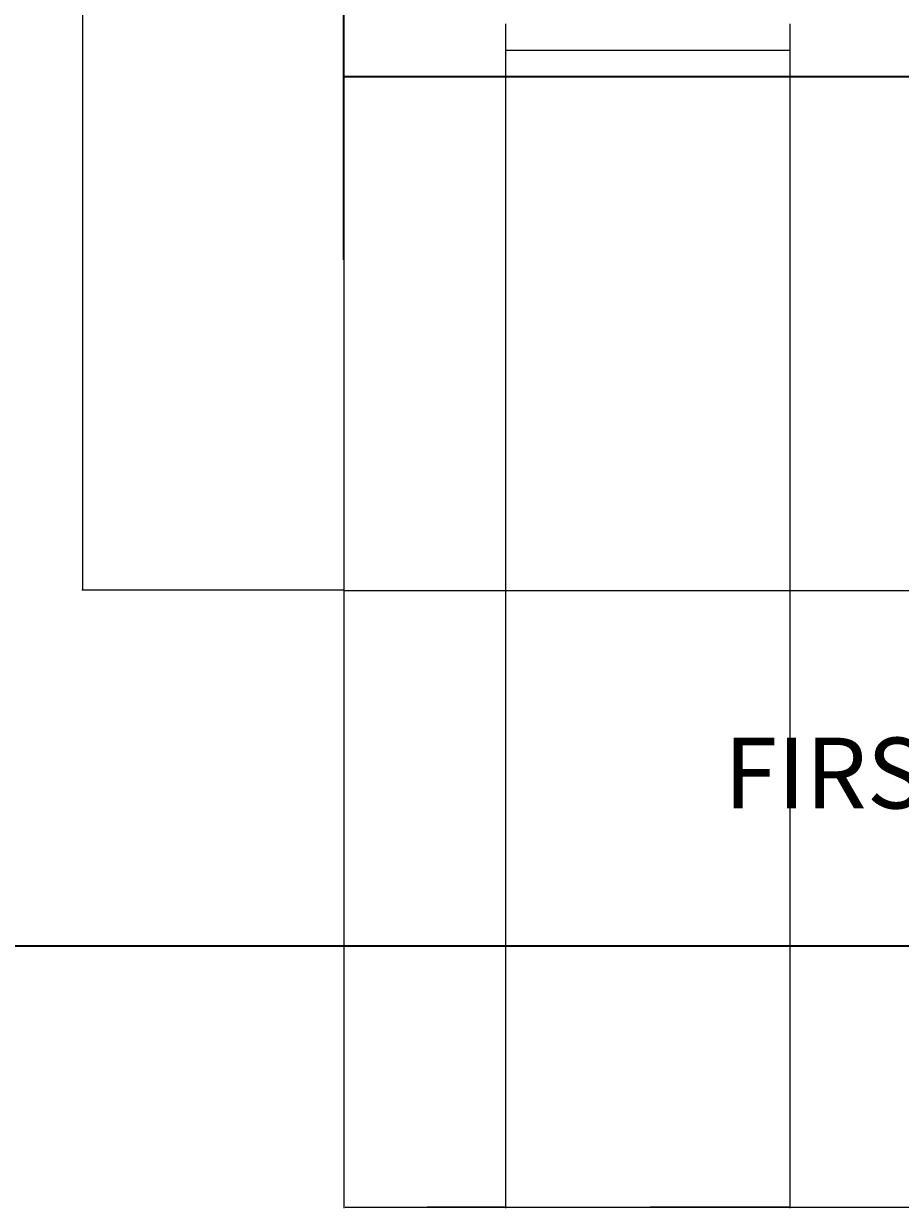
# Model space of a CAD drawing. Units: feet. Extents: x 2100 to 2836, y 2433 to 3396.
# Tile 2 of 12: x 2468 to 2616, y 2433 to 2634. Entities that reach past the tile are written whole.
import ezdxf

# ---------------------------------------------------------------- set-up
doc = ezdxf.new("R2010")
doc.units = ezdxf.units.FT
for name, color, linetype, lineweight in [('A-ANNO-DIMS', 2, 'Continuous', 18), ('A-ANNO-TITL', 7, 'Continuous', 25), ('A-ANNO-TTLB', 7, 'Continuous', 35), ('A-GLAZ', 4, 'Continuous', 18), ('A-WALL', 7, 'Continuous', 35), ('C-PROP', 8, 'Continuous', 18)]:
    doc.layers.add(name, color=color, linetype=linetype, lineweight=lineweight)
doc.styles.get("Standard").update_dxf_attribs({"font": 'arial.ttf'})
doc.dimstyles.get("Standard").update_dxf_attribs({"dimtxt": 0.18, "dimasz": 0.18, "dimexe": 0.18, "dimexo": 0.0625, "dimgap": 0.09, "dimtad": 0, "dimtih": 1, "dimtoh": 1, "dimdec": 4, "dimzin": 0, "dimdsep": 46, "dimtxsty": 'Standard', "dimcen": 0.09, "dimadec": 0, "dimazin": 0, "dimtfac": 1, "dimtdec": 4, "dimtofl": 0, "dimtmove": 0, "dimatfit": 3, "dimfxl": 1, "dimtolj": 1, "dimtzin": 0, "dimarcsym": 0})

# ---------------------------------------------------------------- blocks, each defined once
blk = doc.blocks.new('*D42')
at = {"layer": 'A-ANNO-DIMS', "color": 0, "lineweight": -2, "transparency": 16777216}
for p, q in [((2521.95, 2537.69), (2521.95, 2433.01)), ((2740.95, 2537.69), (2740.95, 2433.01)), ((2522.13, 2433.19), (2631.16, 2433.19)), ((2740.77, 2433.19), (2631.74, 2433.19))]:
    blk.add_line(p, q, dxfattribs=at)
at = {"layer": 'A-ANNO-DIMS', "color": 0, "transparency": 16777216}
for points in [[(2522.13, 2433.22), (2522.13, 2433.16), (2521.95, 2433.19)], [(2740.77, 2433.22), (2740.77, 2433.16), (2740.95, 2433.19)]]:
    blk.add_solid(points, dxfattribs=at)
at = {"layer": 'Defpoints', "color": 0, "transparency": 16777216}
for p in [(2521.95, 2537.76), (2740.95, 2537.76), (2740.95, 2433.19)]:
    blk.add_point(p, dxfattribs=at)
at = {"layer": 'A-ANNO-DIMS', "color": 0, "transparency": 16777216, "insert": (2631.45, 2433.19), "char_height": 0.18, "attachment_point": 5}
blk.add_mtext('\\A1;219', dxfattribs=at)
blk = doc.blocks.new('*D43')
at = {"layer": 'A-ANNO-DIMS', "color": 0, "lineweight": -2, "transparency": 16777216}
for p, q in [((2521.89, 3321.8), (2477.52, 3321.8)), ((2477.7, 3321.62), (2477.7, 2929.96)), ((2477.7, 2537.94), (2477.7, 2929.6)), ((2521.89, 2537.76), (2477.52, 2537.76))]:
    blk.add_line(p, q, dxfattribs=at)
at = {"layer": 'A-ANNO-DIMS', "color": 0, "transparency": 16777216}
for points in [[(2477.67, 3321.62), (2477.73, 3321.62), (2477.7, 3321.8)], [(2477.67, 2537.94), (2477.73, 2537.94), (2477.7, 2537.76)]]:
    blk.add_solid(points, dxfattribs=at)
at = {"layer": 'Defpoints', "color": 0, "transparency": 16777216}
for p in [(2477.7, 3321.8), (2521.95, 3321.8), (2521.95, 2537.76)]:
    blk.add_point(p, dxfattribs=at)
at = {"layer": 'A-ANNO-DIMS', "color": 0, "transparency": 16777216, "insert": (2477.7, 2929.78), "char_height": 0.18, "attachment_point": 5}
blk.add_mtext('\\A1;784', dxfattribs=at)
blk = doc.blocks.new('*D59')
at = {"layer": 'A-ANNO-DIMS', "color": 0, "lineweight": -2, "transparency": 16777216}
for p, q in [((2521.95, 2624.74), (2521.95, 2433.01)), ((2549.36, 2624.74), (2549.36, 2433.01)), ((2522.13, 2433.19), (2535.27, 2433.19)), ((2549.18, 2433.19), (2536.03, 2433.19))]:
    blk.add_line(p, q, dxfattribs=at)
at = {"layer": 'A-ANNO-DIMS', "color": 0, "transparency": 16777216}
for points in [[(2522.13, 2433.22), (2522.13, 2433.16), (2521.95, 2433.19)], [(2549.18, 2433.22), (2549.18, 2433.16), (2549.36, 2433.19)]]:
    blk.add_solid(points, dxfattribs=at)
at = {"layer": 'Defpoints', "color": 0, "transparency": 16777216}
for p in [(2521.95, 2624.8), (2549.36, 2624.8), (2549.36, 2433.19)]:
    blk.add_point(p, dxfattribs=at)
at = {"layer": 'A-ANNO-DIMS', "color": 0, "transparency": 16777216, "insert": (2535.65, 2433.19), "char_height": 0.18, "attachment_point": 5}
blk.add_mtext('\\A1;27.41', dxfattribs=at)
blk = doc.blocks.new('*D60')
at = {"layer": 'A-ANNO-DIMS', "color": 0, "lineweight": -2, "transparency": 16777216}
for p, q in [((2549.36, 2624.74), (2549.36, 2433.01)), ((2597.55, 2624.74), (2597.55, 2433.01)), ((2549.54, 2433.19), (2573.05, 2433.19)), ((2597.37, 2433.19), (2573.85, 2433.19))]:
    blk.add_line(p, q, dxfattribs=at)
at = {"layer": 'A-ANNO-DIMS', "color": 0, "transparency": 16777216}
for points in [[(2549.54, 2433.22), (2549.54, 2433.16), (2549.36, 2433.19)], [(2597.37, 2433.22), (2597.37, 2433.16), (2597.55, 2433.19)]]:
    blk.add_solid(points, dxfattribs=at)
at = {"layer": 'Defpoints', "color": 0, "transparency": 16777216}
for p in [(2549.36, 2624.8), (2597.55, 2624.8), (2597.55, 2433.19)]:
    blk.add_point(p, dxfattribs=at)
at = {"layer": 'A-ANNO-DIMS', "color": 0, "transparency": 16777216, "insert": (2573.45, 2433.19), "char_height": 0.18, "attachment_point": 5}
blk.add_mtext('\\A1;48.19', dxfattribs=at)

msp = doc.modelspace()

# ---------------------------------------------------------------- linework, layer by layer
at = {"layer": 'A-ANNO-TTLB'}
msp.add_lwpolyline([(2144.0848, 3351.6245), (2791.0561, 3351.6245), (2791.0561, 2477.4373), (2144.0848, 2477.4373)], close=True, dxfattribs=at)
at = {"layer": 'A-GLAZ'}
for p, q in [((2549.3574, 2633.8031), (2549.3574, 2624.8031)), ((2597.5459, 2633.8031), (2597.5459, 2624.8031)), ((2549.3574, 2629.3031), (2597.5459, 2629.3031))]:
    msp.add_line(p, q, dxfattribs=at)
at = {"layer": 'A-WALL'}
for p, q in [((2521.9476, 2593.755), (2521.9476, 3321.8031)), ((2659.1783, 2624.8031), (2521.9476, 2624.8031))]:
    msp.add_line(p, q, dxfattribs=at)
at = {"layer": 'C-PROP'}
for p, q in [((2521.9476, 2593.755), (2521.9476, 2537.755)), ((2521.9476, 2537.755), (2740.9476, 2537.755))]:
    msp.add_line(p, q, dxfattribs=at)

# ---------------------------------------------------------------- texts
at = {"layer": 'A-ANNO-TITL'}
msp.add_text('FIRST FLOOR', height=12, dxfattribs=at).set_placement((2586.3598, 2500.7808))

# ---------------------------------------------------------------- dimensions: what is measured, and where the dimension line sits
at = {"layer": 'A-ANNO-DIMS'}
dim = msp.add_linear_dim(base=(2477.6976, 3321.8031), p1=(2521.9476, 2537.755), p2=(2521.9476, 3321.8031), angle=90, dimstyle='Standard', override={"dimdec": 0, "dimlfac": 1, "dimrnd": 0, "dimzin": 0, "dimdsep": 46, "dimlunit": 2}, dxfattribs=at)
dim.commit()
dim.dimension.update_dxf_attribs({"geometry": '*D43', "text_midpoint": (2477.6976, 2929.7791)})
for base, p1, p2, override, picture, middle in [((2549.3574, 2433.1873), (2521.9476, 2624.8031), (2549.3574, 2624.8031), {"dimdec": 2, "dimlfac": 1, "dimrnd": 0, "dimzin": 0, "dimdsep": 46, "dimlunit": 2}, '*D59', (2535.6525, 2433.1873)), ((2597.5459, 2433.1873), (2549.3574, 2624.8031), (2597.5459, 2624.8031), {"dimdec": 2, "dimlfac": 1, "dimrnd": 0, "dimzin": 0, "dimdsep": 46, "dimlunit": 2}, '*D60', (2573.4517, 2433.1873)), ((2740.9476, 2433.1873), (2521.9476, 2537.755), (2740.9476, 2537.755), {"dimdec": 0, "dimlfac": 1, "dimrnd": 0, "dimzin": 0, "dimdsep": 46, "dimlunit": 2}, '*D42', (2631.4476, 2433.1873))]:
    dim = msp.add_linear_dim(base=base, p1=p1, p2=p2, dimstyle='Standard', override=override, dxfattribs=at)
    dim.commit()
    dim.dimension.update_dxf_attribs({"geometry": picture, "text_midpoint": middle})

doc.saveas('drawing.dxf')
